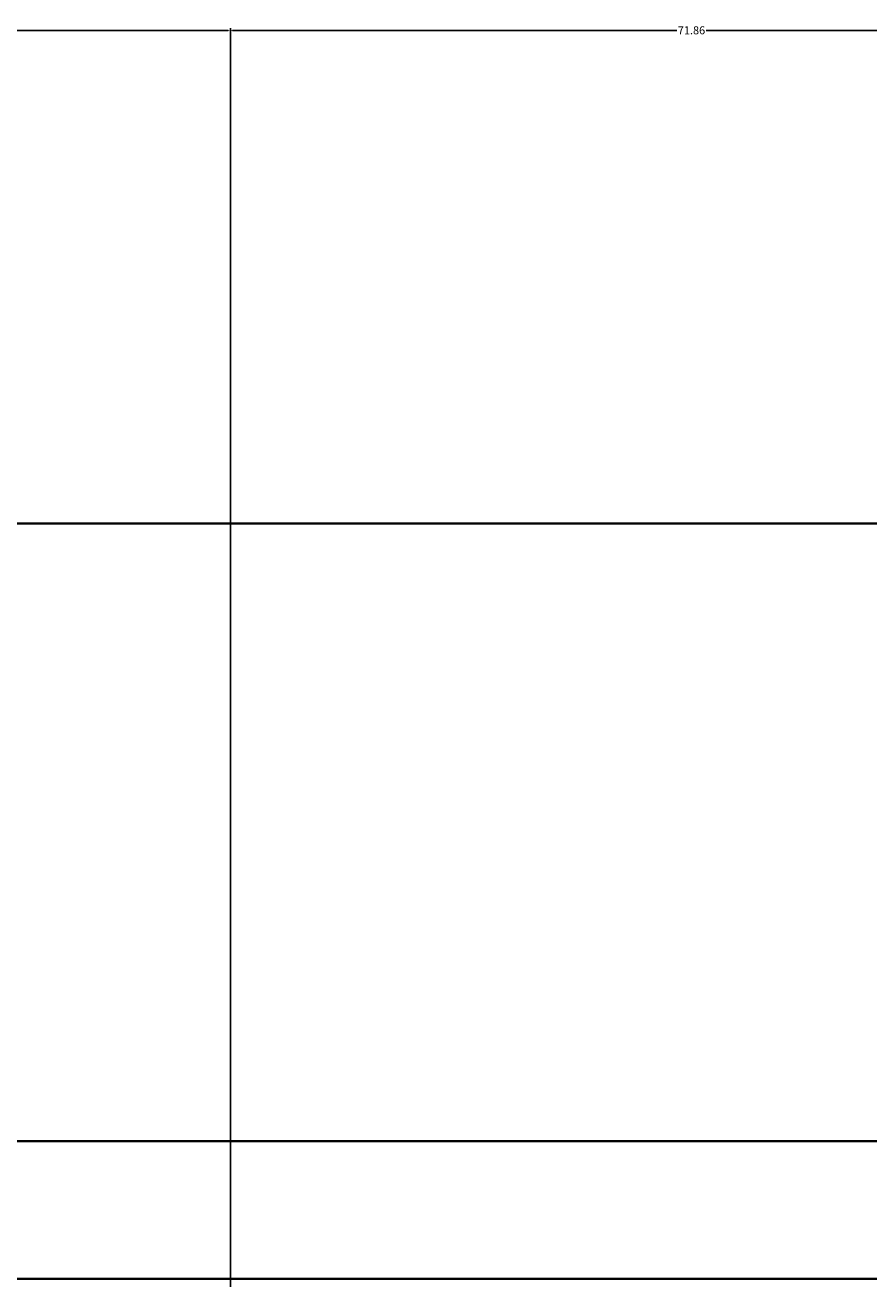
# Model space of a CAD drawing. Units: inches. Extents: x -13 to 809, y 112 to 656.
# Tile 40 of 55: x 455 to 521, y 559 to 656. Entities that reach past the tile are written whole.
import ezdxf

# ---------------------------------------------------------------- set-up
doc = ezdxf.new("R2010")
doc.units = ezdxf.units.IN
doc.header["$MEASUREMENT"] = 0
doc.layers.add('A-ANNO-DIMS', color=2, linetype='Continuous', lineweight=18)
doc.layers.add('A-ELEV', color=7, linetype='Continuous', lineweight=35)
doc.styles.get("Standard").update_dxf_attribs({"font": 'arial.ttf'})
doc.dimstyles.get("Standard").update_dxf_attribs({"dimtxt": 0.625, "dimasz": 0.18, "dimexe": 0.18, "dimexo": 0.0625, "dimgap": 0.09, "dimtad": 0, "dimtih": 1, "dimtoh": 1, "dimdec": 4, "dimzin": 0, "dimdsep": 46, "dimlunit": 4, "dimtxsty": 'Standard', "dimcen": 0.09, "dimadec": 0, "dimazin": 0, "dimtfac": 1, "dimtdec": 4, "dimtofl": 0, "dimtmove": 0, "dimatfit": 3, "dimfxl": 1, "dimtolj": 1, "dimtzin": 0, "dimarcsym": 0})

# ---------------------------------------------------------------- blocks, each defined once
blk = doc.blocks.new('*D26')
at = {"layer": 'A-ANNO-DIMS', "color": 0, "lineweight": -2, "transparency": 16777216}
for p, q in [((341.407, 524.343), (341.407, 655.963)), ((341.587, 655.783), (405.138, 655.783)), ((470.92, 655.783), (407.369, 655.783)), ((471.1, 470.939), (471.1, 655.963))]:
    blk.add_line(p, q, dxfattribs=at)
at = {"layer": 'A-ANNO-DIMS', "color": 0, "transparency": 16777216}
for points in [[(341.587, 655.813), (341.587, 655.753), (341.407, 655.783)], [(470.92, 655.813), (470.92, 655.753), (471.1, 655.783)]]:
    blk.add_solid(points, dxfattribs=at)
at = {"layer": 'Defpoints', "color": 0, "transparency": 16777216}
for p in [(471.1, 655.783), (341.407, 524.281), (471.1, 470.877)]:
    blk.add_point(p, dxfattribs=at)
at = {"layer": 'A-ANNO-DIMS', "color": 0, "transparency": 16777216, "insert": (406.253, 655.783), "char_height": 0.625, "attachment_point": 5}
blk.add_mtext('\\A1;129.7', dxfattribs=at)
blk = doc.blocks.new('*D27')
at = {"layer": 'A-ANNO-DIMS', "color": 0, "lineweight": -2, "transparency": 16777216}
for p, q in [((471.1, 470.939), (471.1, 655.963)), ((471.28, 655.783), (505.889, 655.783)), ((542.782, 655.783), (508.173, 655.783)), ((542.962, 524.343), (542.962, 655.963))]:
    blk.add_line(p, q, dxfattribs=at)
at = {"layer": 'A-ANNO-DIMS', "color": 0, "transparency": 16777216}
for points in [[(471.28, 655.813), (471.28, 655.753), (471.1, 655.783)], [(542.782, 655.813), (542.782, 655.753), (542.962, 655.783)]]:
    blk.add_solid(points, dxfattribs=at)
at = {"layer": 'Defpoints', "color": 0, "transparency": 16777216}
for p in [(542.962, 655.783), (542.962, 524.281), (471.1, 470.877)]:
    blk.add_point(p, dxfattribs=at)
at = {"layer": 'A-ANNO-DIMS', "color": 0, "transparency": 16777216, "insert": (507.031, 655.783), "char_height": 0.625, "attachment_point": 5}
blk.add_mtext('\\A1;71.86', dxfattribs=at)

msp = doc.modelspace()

# ---------------------------------------------------------------- linework, layer by layer
at = {"layer": 'A-ELEV'}
for p, q in [((311.6991, 617.3708), (621.008, 617.3708)), ((292.923, 569.2414), (644.6221, 569.2414)), ((341.4072, 558.5199), (591.008, 558.5199))]:
    msp.add_line(p, q, dxfattribs=at)

# ---------------------------------------------------------------- dimensions: what is measured, and where the dimension line sits
at = {"layer": 'A-ANNO-DIMS'}
for base, p1, p2, override, picture, middle in [((471.0998, 655.7828), (341.4072, 524.281), (471.0998, 470.8765), {"dimdec": 1, "dimlfac": 1, "dimrnd": 0, "dimzin": 0, "dimdsep": 46, "dimlunit": 2}, '*D26', (406.2535, 655.7828)), ((542.9617, 655.7828), (471.0998, 470.8765), (542.9617, 524.281), {"dimdec": 2, "dimlfac": 1, "dimrnd": 0, "dimzin": 0, "dimdsep": 46, "dimlunit": 2}, '*D27', (507.0308, 655.7828))]:
    dim = msp.add_linear_dim(base=base, p1=p1, p2=p2, dimstyle='Standard', override=override, dxfattribs=at)
    dim.commit()
    dim.dimension.update_dxf_attribs({"geometry": picture, "text_midpoint": middle})

doc.saveas('drawing.dxf')
